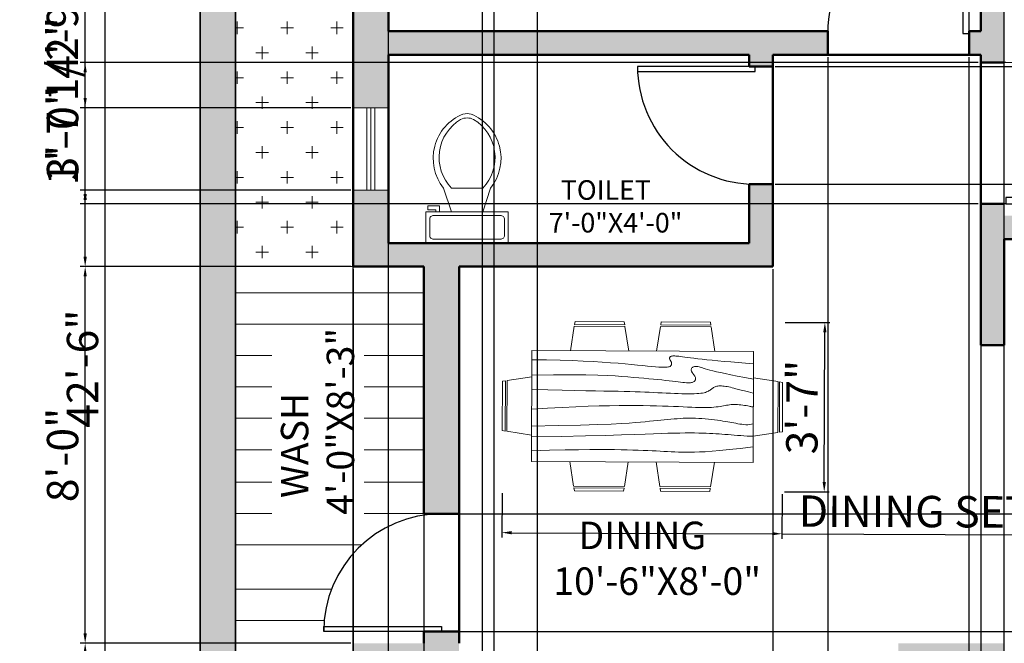
# Model space of a CAD drawing. Units: inches. Extents: x 1369 to 1844, y 2136 to 2743.
# Tile 2 of 4: x 1369 to 1620, y 2358 to 2517. Entities that reach past the tile are written whole.
import ezdxf

# ---------------------------------------------------------------- set-up
doc = ezdxf.new("R2010")
doc.units = ezdxf.units.IN
for name, color, linetype, lineweight in [('A-ANNO-DIMS', 2, 'Continuous', 18), ('A-AREA-IDEN', 7, 'Continuous', 25), ('A-DOOR', 4, 'Continuous', 25), ('A-FLOR-FIXT', 9, 'Continuous', 20), ('A-FLOR-PATT', 9, 'Continuous', 13), ('A-FURN', 8, 'Continuous', 18), ('A-WALL', 7, 'Continuous', 50), ('C-PROP', 7, 'Continuous', 35), ('L-PLNT', 3, 'Continuous', 18)]:
    doc.layers.add(name, color=color, linetype=linetype, lineweight=lineweight)
for name, color, linetype, lineweight, true_color in [('A-GLAZ', 244, 'Continuous', 20, 0x991b1e), ('A-WALL-PATT', 251, 'Continuous', 13, 0x636466), ('C-PROP-PATT', 251, 'Continuous', 13, 0x636466), ('L-PLNT-PATT', 116, 'Continuous', 13, 0x136734)]:
    doc.layers.add(name, color=color, linetype=linetype, lineweight=lineweight, true_color=true_color)
doc.styles.get("Standard").update_dxf_attribs({"font": 'arial.ttf'})
doc.dimstyles.new('ISO-25', dxfattribs={"dimtxt": 8, "dimasz": 2.5, "dimexe": 1.25, "dimexo": 0.625, "dimtad": 1, "dimlunit": 3, "dimtxsty": 'Standard', "dimcen": 2.5, "dimadec": 0, "dimazin": 0, "dimtfac": 1, "dimtmove": 0, "dimatfit": 3, "dimfxl": 1, "dimarcsym": 0})

# ---------------------------------------------------------------- blocks, each defined once
blk = doc.blocks.new('*U2')
for p, q in [((0, 0), (0, -6)), ((-40, 0), (-40, -6))]:
    blk.add_line(p, q)
blk.add_lwpolyline([(0, 0), (0, 40), (-1.75, 40), (-1.75, 0)], close=True)
blk.add_arc((0, 0), 40, 90, 180)
blk = doc.blocks.new('*U3')
for p, q in [((0, 0), (0, 6)), ((40, 0), (40, 6))]:
    blk.add_line(p, q)
blk.add_lwpolyline([(0, 0), (0, -40), (1.75, -40), (1.75, 0)], close=True)
blk.add_arc((0, 0), 40, 270, 360)
blk = doc.blocks.new('*U5')
for p, q in [((-40, 0), (-40, 6)), ((0, 0), (0, 6))]:
    blk.add_line(p, q)
blk.add_lwpolyline([(0, 0), (0, -40), (-1.75, -40), (-1.75, 0)], close=True)
blk.add_arc((0, 0), 40, 180, 270)
blk = doc.blocks.new('*U8')
for p, q in [((9.5, -6), (9.5, -2)), ((-10, -8.5), (-8, -8.5)), ((-10, -9.5), (-10, -8.5)), ((-7, -9.5), (-10, -9.5)), ((-8, -8.5), (-8, -8)), ((-7, -8), (-7, -9.5)), ((-4, -8), (-6, -14)), ((4, -8), (6, -14)), ((4, -14), (-4, -14))]:
    blk.add_line(p, q)
blk.add_lwpolyline([(10.5, -8), (10.5, 0), (-10.5, 0), (-10.5, -8)], close=True)
for points in [[(-9.5, -2), (-9.5, -6)], [(8.5, -1), (-8.5, -1)], [(-8.5, -7), (8.5, -7)]]:
    blk.add_lwpolyline(points)
for centre, radius, start, end in [((-8.62, -1.88), 0.884, 81.8699, 188.1301), ((8.62, -1.88), 0.884, 351.8699, 98.1301), ((-8.62, -6.12), 0.884, 171.8699, 278.1301), ((8.62, -6.12), 0.884, 261.8699, 8.1301), ((3.52, -21.58), 12.17, 141.4691, 247.9714), ((4.2, -21.82), 11.33, 136.3677, 238.9468), ((-3.52, -21.58), 12.17, 292.0284, 38.5307), ((-4.2, -21.82), 11.33, 301.053, 43.6321), ((0, -27.88), 4, 245.7318, 294.2682), ((0, -29), 4, 254.8605, 285.1395)]:
    blk.add_arc(centre, radius, start, end)
blk = doc.blocks.new('Dining Set - 36 x 72 in.')
for p, q in [((-22.2343, 26.00059), (-23.4847, 17.99762)), ((-22.2304, 26), (-5.7608, 26)), ((-22, 27.5), (-22.1562, 26.50042)), ((-5.8416, 26.5), (-22.1534, 26.5)), ((-22, 27.5), (-6, 27.5)), ((-5.8437, 26.49966), (-6, 27.5)), ((-4.5152, 17.99762), (-5.7655, 25.99926)), ((5.7657, 26.00059), (4.5153, 17.99762)), ((5.7696, 26), (22.2392, 26)), ((6, 27.5), (5.8438, 26.50042)), ((22.1584, 26.5), (5.8466, 26.5)), ((6, 27.5), (22, 27.5)), ((22.1563, 26.49966), (22, 27.5)), ((23.4848, 17.99762), (22.2345, 25.99926)), ((36, 18), (-36, 18)), ((-36, 18), (-36, -18)), ((36, -18), (36, 18)), ((-45.5, 8), (-44.5004, 8.15617)), ((-45.5, 8), (-45.5, -8)), ((-44.5, -8.15843), (-44.5, 8.15338)), ((-44.0006, 8.23428), (-35.9976, 9.48474)), ((-44, 8.23041), (-44, -8.23915)), ((44.0006, 8.23428), (35.9976, 9.48474)), ((44, 8.23041), (44, -8.23915)), ((44.5, -8.15843), (44.5, 8.15338)), ((45.5, 8), (44.5005, 8.15617)), ((45.5, 8), (45.5, -8)), ((-44.4997, -8.15631), (-45.5, -8)), ((-35.9976, -9.48476), (-43.9993, -8.2345)), ((35.9976, -9.48476), (43.9993, -8.2345)), ((44.4997, -8.15631), (45.5, -8)), ((-36, -18), (36, -18)), ((-22.2343, -26.0006), (-23.4847, -17.99762)), ((-4.5152, -17.99762), (-5.7655, -25.99928)), ((5.7657, -26.0006), (4.5153, -17.99762)), ((23.4848, -17.99762), (22.2345, -25.99928)), ((-22.2304, -26), (-5.7608, -26)), ((-22, -27.5), (-22.1562, -26.50044)), ((-5.8416, -26.5), (-22.1534, -26.5)), ((-22, -27.5), (-6, -27.5)), ((-5.8437, -26.49967), (-6, -27.5)), ((5.7696, -26), (22.2392, -26)), ((6, -27.5), (5.8438, -26.50044)), ((22.1584, -26.5), (5.8466, -26.5)), ((6, -27.5), (22, -27.5)), ((22.1563, -26.49967), (22, -27.5))]:
    blk.add_line(p, q)
for points in [[(-36, 15), (-31.1772, 14.97754), (-26.8079, 14.91406), (-22.8538, 14.81543), (-19.276, 14.6875), (-16.0362, 14.53613), (-13.0957, 14.36718), (-10.4159, 14.18652), (-7.9583, 14), (-5.6904, 13.81315), (-3.6035, 13.63021), (-1.6954, 13.45508), (0.0365, 13.29166), (1.5945, 13.14388), (2.9811, 13.01562), (4.1988, 12.9108), (5.25, 12.83333), (6.1393, 12.78613), (6.8802, 12.76823), (7.4883, 12.77767), (7.9792, 12.8125), (8.3685, 12.87077), (8.6719, 12.95052), (8.9049, 13.0498), (9.0833, 13.16666), (9.2205, 13.29899), (9.3216, 13.44401), (9.3895, 13.59879), (9.4271, 13.76041), (9.4373, 13.92594), (9.4232, 14.09245), (9.3875, 14.257), (9.3333, 14.41666), (9.2638, 14.56917), (9.1836, 14.71484), (9.0975, 14.85465), (9.0104, 14.98958), (8.9272, 15.1206), (8.8529, 15.2487), (8.7922, 15.37483), (8.75, 15.5), (8.7305, 15.62467), (8.7344, 15.74739), (8.7617, 15.86621), (8.8125, 15.97916), (8.8867, 16.08431), (8.9844, 16.17968), (9.1055, 16.26334), (9.25, 16.33333), (9.4189, 16.38802), (9.6172, 16.42708), (9.8506, 16.45052), (10.125, 16.45833), (10.4463, 16.45052), (10.8203, 16.42708), (11.2529, 16.38802), (11.75, 16.33333), (12.3184, 16.26318), (12.9694, 16.17838), (13.7151, 16.07991), (14.5677, 15.96875), (15.5395, 15.84586), (16.6426, 15.71224), (17.8893, 15.56884), (19.2917, 15.41666), (20.859, 15.25667), (22.5879, 15.08984), (24.4721, 14.91715), (26.5052, 14.73958), (28.6809, 14.5581), (30.9929, 14.3737), (33.4347, 14.18733), (36, 14)], [(-36, 10), (-28.9766, 10.14274), (-23.1725, 10.20442), (-18.4241, 10.19775), (-14.5677, 10.13541), (-11.4399, 10.03011), (-8.877, 9.89453), (-6.7154, 9.74137), (-4.7917, 9.58333), (-2.9698, 9.43082), (-1.2246, 9.28515), (0.4415, 9.14534), (2.026, 9.01041), (3.5266, 8.87939), (4.9408, 8.7513), (6.266, 8.62516), (7.5, 8.5), (8.6411, 8.37549), (9.6914, 8.2539), (10.6538, 8.13818), (11.5312, 8.03125), (12.3267, 7.93603), (13.043, 7.85547), (13.6831, 7.79248), (14.25, 7.75), (14.7471, 7.7303), (15.1797, 7.73307), (15.5537, 7.75732), (15.875, 7.80208), (16.1494, 7.86637), (16.3828, 7.94922), (16.5811, 8.04964), (16.75, 8.16666), (16.8944, 8.29915), (17.0143, 8.44531), (17.1089, 8.60319), (17.1771, 8.77083), (17.218, 8.94629), (17.2305, 9.1276), (17.2137, 9.31282), (17.1667, 9.5), (17.0895, 9.6875), (16.987, 9.875), (16.8649, 10.0625), (16.7292, 10.25), (16.5856, 10.4375), (16.4401, 10.625), (16.2985, 10.8125), (16.1667, 11), (16.05, 11.18733), (15.9518, 11.3737), (15.8752, 11.5581), (15.8229, 11.73958), (15.798, 11.91715), (15.8034, 12.08984), (15.842, 12.25667), (15.9167, 12.41666), (16.0295, 12.56836), (16.1784, 12.70833), (16.3605, 12.83268), (16.5729, 12.9375), (16.8127, 13.01888), (17.0768, 13.07291), (17.3625, 13.0957), (17.6667, 13.08333), (17.9894, 13.03312), (18.3418, 12.94726), (18.7382, 12.82918), (19.1927, 12.68229), (19.7195, 12.51001), (20.3327, 12.31575), (21.0465, 12.10294), (21.875, 11.875), (22.8357, 11.63354), (23.959, 11.37304), (25.2786, 11.08618), (26.8282, 10.76562), (28.6414, 10.40405), (30.752, 9.99414), (33.1936, 9.52856), (36, 9)], [(-36, 5.5), (-30.7157, 5.3348), (-26.069, 5.20963), (-21.9946, 5.11767), (-18.4271, 5.05208), (-15.3009, 5.00602), (-12.5508, 4.97265), (-10.1112, 4.94515), (-7.9167, 4.91666), (-5.909, 4.88167), (-4.0586, 4.83984), (-2.3429, 4.79215), (-0.7396, 4.73958), (0.7739, 4.6831), (2.22, 4.6237), (3.6213, 4.56233), (5, 4.5), (6.373, 4.43782), (7.7344, 4.3776), (9.0723, 4.32129), (10.375, 4.27083), (11.6309, 4.22819), (12.8281, 4.19531), (13.9551, 4.17415), (15, 4.16666), (15.954, 4.17448), (16.819, 4.19791), (17.6001, 4.23698), (18.3021, 4.29166), (18.9299, 4.36198), (19.4883, 4.44791), (19.9823, 4.54948), (20.4167, 4.66666), (20.7969, 4.79899), (21.1302, 4.94401), (21.4245, 5.09879), (21.6875, 5.26041), (21.9271, 5.42594), (22.1511, 5.59245), (22.3672, 5.757), (22.5834, 5.91666), (22.8065, 6.06868), (23.0404, 6.21093), (23.2879, 6.34147), (23.5521, 6.45833), (23.8358, 6.55957), (24.142, 6.64323), (24.4735, 6.70735), (24.8334, 6.75), (25.2235, 6.76969), (25.642, 6.76692), (26.0858, 6.74267), (26.5521, 6.69791), (27.0379, 6.63362), (27.5404, 6.55078), (28.0565, 6.45036), (28.5834, 6.33333), (29.1242, 6.19987), (29.7071, 6.04687), (30.3661, 5.87044), (31.1354, 5.66666), (32.0493, 5.43164), (33.142, 5.16146), (34.4475, 4.85221), (36, 4.5)], [(-36, -1), (-30.7915, -0.6591), (-26.0195, -0.38216), (-21.6519, -0.16284), (-17.6563, 0.00521), (-14.0005, 0.12833), (-10.6523, 0.21289), (-7.5796, 0.26522), (-4.75, 0.29166), (-2.134, 0.29793), (0.2878, 0.28711), (2.5317, 0.26163), (4.6146, 0.22396), (6.5529, 0.17651), (8.3633, 0.12174), (10.0623, 0.06209), (11.6667, 0), (13.1899, -0.06201), (14.6341, -0.1211), (15.9982, -0.17432), (17.2813, -0.21875), (18.4823, -0.25147), (19.6003, -0.26953), (20.6343, -0.27002), (21.5834, -0.25), (22.4481, -0.20768), (23.2357, -0.14584), (23.9549, -0.06836), (24.6146, 0.02083), (25.2235, 0.11784), (25.7904, 0.21875), (26.3241, 0.31966), (26.8334, 0.41666), (27.3265, 0.50618), (27.8099, 0.58593), (28.2894, 0.65397), (28.7709, 0.70833), (29.2601, 0.74707), (29.763, 0.76823), (30.2855, 0.76985), (30.8334, 0.75), (31.4088, 0.70784), (31.9994, 0.64713), (32.589, 0.57275), (33.1615, 0.48958), (33.7008, 0.4025), (34.1908, 0.3164), (34.6153, 0.23616), (34.9584, 0.16666), (35.2099, 0.11165), (35.3848, 0.07031), (35.504, 0.04069), (35.5886, 0.02083), (35.6594, 0.00879), (35.7377, 0.0026), (35.8442, 0.00032), (36, 0)], [(-36, -6.5), (-27.1843, -6.31267), (-20.084, -6.1263), (-14.469, -5.9419), (-10.1094, -5.76042), (-6.7752, -5.58285), (-4.2363, -5.41016), (-2.2629, -5.24333), (-0.625, -5.08334), (0.8708, -4.93099), (2.2715, -4.78646), (3.5872, -4.64974), (4.8281, -4.52084), (6.0046, -4.39974), (7.127, -4.28646), (8.2053, -4.18099), (9.25, -4.08334), (10.2705, -3.99382), (11.2734, -3.91407), (12.2647, -3.84603), (13.25, -3.79167), (14.2354, -3.75293), (15.2266, -3.73177), (16.2295, -3.73015), (17.25, -3.75), (18.2912, -3.79248), (19.3451, -3.85547), (20.4009, -3.93604), (21.4479, -4.03125), (22.4754, -4.13819), (23.4727, -4.25391), (24.4289, -4.37549), (25.3334, -4.5), (26.1785, -4.62492), (26.9694, -4.74935), (27.7145, -4.87281), (28.4219, -4.99479), (29.1, -5.11483), (29.7572, -5.23242), (30.4016, -5.34709), (31.0417, -5.45834), (31.6837, -5.56437), (32.3262, -5.65821), (32.9658, -5.73153), (33.599, -5.77604), (34.2224, -5.78345), (34.8327, -5.74545), (35.4264, -5.65373), (36, -5.5)], [(-36, -10), (-26.4022, -9.81299), (-18.4675, -9.62891), (-11.9839, -9.45069), (-6.7396, -9.28125), (-2.5226, -9.12354), (0.8789, -8.98047), (3.6769, -8.85498), (6.0833, -8.75), (8.2767, -8.66765), (10.3021, -8.60677), (12.1712, -8.56543), (13.8958, -8.54167), (15.4876, -8.53353), (16.9583, -8.53907), (18.3197, -8.55632), (19.5834, -8.58334), (20.7616, -8.61841), (21.8685, -8.66081), (22.9188, -8.71004), (23.9271, -8.76563), (24.9081, -8.82707), (25.8763, -8.89388), (26.8465, -8.96558), (27.8334, -9.04167), (28.8474, -9.12118), (29.8828, -9.20117), (30.93, -9.27824), (31.9792, -9.34896), (33.0205, -9.40991), (34.0443, -9.45768), (35.0407, -9.48885), (36, -9.5)], [(-36, -14.5), (-30.0881, -14.33513), (-25.0332, -14.21224), (-20.7312, -14.12647), (-17.0781, -14.07292), (-13.97, -14.04671), (-11.3027, -14.04297), (-8.9724, -14.05681), (-6.875, -14.08334), (-4.9224, -14.11833), (-3.0905, -14.16016), (-1.3709, -14.20785), (0.2448, -14.26042), (1.7647, -14.3169), (3.1973, -14.3763), (4.5507, -14.43767), (5.8333, -14.5), (7.0554, -14.5621), (8.235, -14.62175), (9.3922, -14.67652), (10.5469, -14.72396), (11.7192, -14.76164), (12.929, -14.78711), (14.1965, -14.79794), (15.5417, -14.79167), (16.9933, -14.76424), (18.6152, -14.70508), (20.4804, -14.60197), (22.6615, -14.44271), (25.2312, -14.21509), (28.2624, -13.9069), (31.8277, -13.50594), (36, -13)]]:
    blk.add_lwpolyline(points)
blk = doc.blocks.new('*D12')
at = {"layer": 'A-ANNO-DIMS', "color": 0, "lineweight": -2, "transparency": 16777216}
for p, q in [((1413.89, 2682.76), (1389.03, 2682.76)), ((1390.28, 2175.26), (1390.28, 2680.26)), ((1413.89, 2172.76), (1389.03, 2172.76))]:
    blk.add_line(p, q, dxfattribs=at)
at = {"layer": 'A-ANNO-DIMS', "color": 0, "transparency": 16777216}
for points in [[(1389.86, 2680.26), (1390.69, 2680.26), (1390.28, 2682.76)], [(1389.86, 2175.26), (1390.69, 2175.26), (1390.28, 2172.76)]]:
    blk.add_solid(points, dxfattribs=at)
at = {"layer": 'Defpoints', "color": 0, "transparency": 16777216}
for p in [(1390.28, 2682.76), (1414.51, 2682.76), (1414.51, 2172.76)]:
    blk.add_point(p, dxfattribs=at)
at = {"layer": 'A-ANNO-DIMS', "color": 0, "transparency": 16777216, "insert": (1385.57, 2427.76), "char_height": 8, "attachment_point": 5, "rotation": 90}
blk.add_mtext('42\'-6"', dxfattribs=at)
blk = doc.blocks.new('WIN-21IN')
for p, q in [((3.5, 21), (3.5, 0)), ((4.5, 21), (4.5, 0)), ((5.5, 21), (5.5, 0))]:
    blk.add_line(p, q)
blk.add_lwpolyline([(0, 21), (9, 21), (9, 0), (0, 0)], close=True)
blk = doc.blocks.new('*D24')
at = {"layer": 'A-ANNO-DIMS', "color": 0, "lineweight": -2, "transparency": 16777216}
for p, q in [((1491.47, 2396.04), (1491.42, 2384.71)), ((1562.89, 2395.76), (1562.84, 2384.42)), ((1493.93, 2385.95), (1560.35, 2385.68)), ((1562.85, 2385.67), (1679.38, 2385.22))]:
    blk.add_line(p, q, dxfattribs=at)
at = {"layer": 'A-ANNO-DIMS', "color": 0, "transparency": 16777216}
for points in [[(1493.93, 2386.36), (1493.93, 2385.53), (1491.43, 2385.96)], [(1560.35, 2386.1), (1560.35, 2385.27), (1562.85, 2385.67)]]:
    blk.add_solid(points, dxfattribs=at)
at = {"layer": 'Defpoints', "color": 0, "transparency": 16777216}
for p in [(1491.47, 2396.67), (1562.89, 2396.39), (1562.85, 2385.67)]:
    blk.add_point(p, dxfattribs=at)
at = {"layer": 'A-ANNO-DIMS', "color": 0, "transparency": 16777216, "insert": (1622.38, 2390.2), "char_height": 8, "attachment_point": 5, "rotation": 359.7742}
blk.add_mtext('DINING SET 5\'-11 1/2"', dxfattribs=at)
blk = doc.blocks.new('*D25')
at = {"layer": 'A-ANNO-DIMS', "color": 0, "lineweight": -2, "transparency": 16777216}
for p, q in [((1563.69, 2439.55), (1575.02, 2439.51)), ((1573.61, 2398.85), (1573.76, 2437.01)), ((1563.52, 2396.38), (1574.85, 2396.34))]:
    blk.add_line(p, q, dxfattribs=at)
at = {"layer": 'A-ANNO-DIMS', "color": 0, "transparency": 16777216}
for points in [[(1573.35, 2437.01), (1574.18, 2437.01), (1573.77, 2439.51)], [(1573.2, 2398.85), (1574.03, 2398.84), (1573.6, 2396.35)]]:
    blk.add_solid(points, dxfattribs=at)
at = {"layer": 'Defpoints', "color": 0, "transparency": 16777216}
for p in [(1563.06, 2439.55), (1573.77, 2439.51), (1562.89, 2396.39)]:
    blk.add_point(p, dxfattribs=at)
at = {"layer": 'A-ANNO-DIMS', "color": 0, "transparency": 16777216, "insert": (1568.98, 2417.95), "char_height": 8, "attachment_point": 5, "rotation": 89.7742}
blk.add_mtext('3\'-7"', dxfattribs=at)
blk = doc.blocks.new('*D37')
at = {"layer": 'A-ANNO-DIMS', "color": 0, "lineweight": -2, "transparency": 16777216}
for p, q in [((1452.89, 2357.76), (1383.96, 2357.76)), ((1385.21, 2261.26), (1385.21, 2355.26)), ((1452.89, 2258.76), (1383.96, 2258.76))]:
    blk.add_line(p, q, dxfattribs=at)
at = {"layer": 'A-ANNO-DIMS', "color": 0, "transparency": 16777216}
for points in [[(1384.79, 2355.26), (1385.63, 2355.26), (1385.21, 2357.76)], [(1384.79, 2261.26), (1385.63, 2261.26), (1385.21, 2258.76)]]:
    blk.add_solid(points, dxfattribs=at)
at = {"layer": 'Defpoints', "color": 0, "transparency": 16777216}
for p in [(1385.21, 2357.76), (1453.51, 2357.76), (1453.51, 2258.76)]:
    blk.add_point(p, dxfattribs=at)
at = {"layer": 'A-ANNO-DIMS', "color": 0, "transparency": 16777216, "insert": (1380.5, 2308.26), "char_height": 8, "attachment_point": 5, "rotation": 90}
blk.add_mtext('8\'-3"', dxfattribs=at)
blk = doc.blocks.new('*D38')
at = {"layer": 'A-ANNO-DIMS', "color": 0, "lineweight": -2, "transparency": 16777216}
for p, q in [((1452.89, 2453.76), (1383.96, 2453.76)), ((1385.21, 2360.26), (1385.21, 2451.26)), ((1452.89, 2357.76), (1383.96, 2357.76))]:
    blk.add_line(p, q, dxfattribs=at)
at = {"layer": 'A-ANNO-DIMS', "color": 0, "transparency": 16777216}
for points in [[(1384.79, 2451.26), (1385.63, 2451.26), (1385.21, 2453.76)], [(1384.79, 2360.26), (1385.63, 2360.26), (1385.21, 2357.76)]]:
    blk.add_solid(points, dxfattribs=at)
at = {"layer": 'Defpoints', "color": 0, "transparency": 16777216}
for p in [(1385.21, 2453.76), (1453.51, 2453.76), (1453.51, 2357.76)]:
    blk.add_point(p, dxfattribs=at)
at = {"layer": 'A-ANNO-DIMS', "color": 0, "transparency": 16777216, "insert": (1380.5, 2405.76), "char_height": 8, "attachment_point": 5, "rotation": 90}
blk.add_mtext('8\'-0"', dxfattribs=at)
blk = doc.blocks.new('*D39')
at = {"layer": 'A-ANNO-DIMS', "color": 0, "lineweight": -2, "transparency": 16777216}
for p, q in [((1385.21, 2473.26), (1385.21, 2516.16)), ((1452.89, 2473.26), (1383.96, 2473.26)), ((1385.21, 2456.26), (1385.21, 2470.76)), ((1452.89, 2453.76), (1383.96, 2453.76))]:
    blk.add_line(p, q, dxfattribs=at)
at = {"layer": 'A-ANNO-DIMS', "color": 0, "transparency": 16777216}
for points in [[(1384.79, 2470.76), (1385.63, 2470.76), (1385.21, 2473.26)], [(1384.79, 2456.26), (1385.63, 2456.26), (1385.21, 2453.76)]]:
    blk.add_solid(points, dxfattribs=at)
at = {"layer": 'Defpoints', "color": 0, "transparency": 16777216}
for p in [(1385.21, 2473.26), (1453.51, 2473.26), (1453.51, 2453.76)]:
    blk.add_point(p, dxfattribs=at)
at = {"layer": 'A-ANNO-DIMS', "color": 0, "transparency": 16777216, "insert": (1380.45, 2495.96), "char_height": 8, "attachment_point": 5, "rotation": 90}
blk.add_mtext('1\'-7 1/2"', dxfattribs=at)
blk = doc.blocks.new('*D40')
at = {"layer": 'A-ANNO-DIMS', "color": 0, "lineweight": -2, "transparency": 16777216}
for p, q in [((1452.89, 2551.88), (1383.96, 2551.88)), ((1385.21, 2496.76), (1385.21, 2549.38)), ((1452.89, 2494.26), (1383.96, 2494.26))]:
    blk.add_line(p, q, dxfattribs=at)
at = {"layer": 'A-ANNO-DIMS', "color": 0, "transparency": 16777216}
for points in [[(1384.79, 2549.38), (1385.63, 2549.38), (1385.21, 2551.88)], [(1384.79, 2496.76), (1385.63, 2496.76), (1385.21, 2494.26)]]:
    blk.add_solid(points, dxfattribs=at)
at = {"layer": 'Defpoints', "color": 0, "transparency": 16777216}
for p in [(1385.21, 2551.88), (1453.51, 2551.88), (1453.51, 2494.26)]:
    blk.add_point(p, dxfattribs=at)
at = {"layer": 'A-ANNO-DIMS', "color": 0, "transparency": 16777216, "insert": (1380.45, 2523.07), "char_height": 8, "attachment_point": 5, "rotation": 90}
blk.add_mtext('4\'-9 1/2"', dxfattribs=at)
blk = doc.blocks.new('*D42')
at = {"layer": 'A-ANNO-DIMS', "color": 0, "lineweight": -2, "transparency": 16777216}
for p, q in [((1453.51, 2453.13), (1453.51, 2142.21)), ((1471.51, 2453.13), (1471.51, 2142.21)), ((1456.01, 2143.46), (1469.01, 2143.46)), ((1471.51, 2143.46), (1495.77, 2143.46))]:
    blk.add_line(p, q, dxfattribs=at)
at = {"layer": 'A-ANNO-DIMS', "color": 0, "transparency": 16777216}
for points in [[(1456.01, 2143.87), (1456.01, 2143.04), (1453.51, 2143.46)], [(1469.01, 2143.87), (1469.01, 2143.04), (1471.51, 2143.46)]]:
    blk.add_solid(points, dxfattribs=at)
at = {"layer": 'Defpoints', "color": 0, "transparency": 16777216}
for p in [(1453.51, 2453.76), (1471.51, 2453.76), (1471.51, 2143.46)]:
    blk.add_point(p, dxfattribs=at)
at = {"layer": 'A-ANNO-DIMS', "color": 0, "transparency": 16777216, "insert": (1484.89, 2148.17), "char_height": 8, "attachment_point": 5}
blk.add_mtext('1\'-6"', dxfattribs=at)
blk = doc.blocks.new('*D45')
at = {"layer": 'A-ANNO-DIMS', "color": 0, "lineweight": -2, "transparency": 16777216}
for p, q in [((1619.51, 2326.38), (1619.51, 2734.31)), ((1636.5, 2326.38), (1636.5, 2734.31)), ((1622.01, 2733.06), (1634, 2733.06)), ((1636.5, 2733.06), (1660.77, 2733.06))]:
    blk.add_line(p, q, dxfattribs=at)
at = {"layer": 'A-ANNO-DIMS', "color": 0, "transparency": 16777216}
for points in [[(1622.01, 2733.47), (1622.01, 2732.64), (1619.51, 2733.06)], [(1634, 2733.47), (1634, 2732.64), (1636.5, 2733.06)]]:
    blk.add_solid(points, dxfattribs=at)
at = {"layer": 'Defpoints', "color": 0, "transparency": 16777216}
for p in [(1636.5, 2733.06), (1619.51, 2325.76), (1636.5, 2325.76)]:
    blk.add_point(p, dxfattribs=at)
at = {"layer": 'A-ANNO-DIMS', "color": 0, "transparency": 16777216, "insert": (1649.88, 2737.77), "char_height": 8, "attachment_point": 5}
blk.add_mtext('1\'-5"', dxfattribs=at)
blk = doc.blocks.new('*D49')
at = {"layer": 'A-ANNO-DIMS', "color": 0, "lineweight": -2, "transparency": 16777216}
for p, q in [((1574.51, 2507.13), (1574.51, 2142.21)), ((1610.51, 2507.13), (1610.51, 2142.21)), ((1577.01, 2143.46), (1608.01, 2143.46))]:
    blk.add_line(p, q, dxfattribs=at)
at = {"layer": 'A-ANNO-DIMS', "color": 0, "transparency": 16777216}
for points in [[(1577.01, 2143.87), (1577.01, 2143.04), (1574.51, 2143.46)], [(1608.01, 2143.87), (1608.01, 2143.04), (1610.51, 2143.46)]]:
    blk.add_solid(points, dxfattribs=at)
at = {"layer": 'Defpoints', "color": 0, "transparency": 16777216}
for p in [(1574.51, 2507.76), (1610.51, 2507.76), (1610.51, 2143.46)]:
    blk.add_point(p, dxfattribs=at)
at = {"layer": 'A-ANNO-DIMS', "color": 0, "transparency": 16777216, "insert": (1592.51, 2148.17), "char_height": 8, "attachment_point": 5}
blk.add_mtext('3\'-0"', dxfattribs=at)
blk = doc.blocks.new('*D50')
at = {"layer": 'A-ANNO-DIMS', "color": 0, "lineweight": -2, "transparency": 16777216}
for p, q in [((1612.89, 2505.76), (1383.96, 2505.76)), ((1385.21, 2472.26), (1385.21, 2503.26)), ((1612.89, 2469.76), (1383.96, 2469.76))]:
    blk.add_line(p, q, dxfattribs=at)
at = {"layer": 'A-ANNO-DIMS', "color": 0, "transparency": 16777216}
for points in [[(1384.79, 2503.26), (1385.63, 2503.26), (1385.21, 2505.76)], [(1384.79, 2472.26), (1385.63, 2472.26), (1385.21, 2469.76)]]:
    blk.add_solid(points, dxfattribs=at)
at = {"layer": 'Defpoints', "color": 0, "transparency": 16777216}
for p in [(1385.21, 2505.76), (1613.51, 2505.76), (1613.51, 2469.76)]:
    blk.add_point(p, dxfattribs=at)
at = {"layer": 'A-ANNO-DIMS', "color": 0, "transparency": 16777216, "insert": (1380.5, 2487.76), "char_height": 8, "attachment_point": 5, "rotation": 90}
blk.add_mtext('3\'-0"', dxfattribs=at)
blk = doc.blocks.new('*D51')
at = {"layer": 'A-ANNO-DIMS', "color": 0, "lineweight": -2, "transparency": 16777216}
for p, q in [((1561.14, 2504.76), (1838.06, 2504.76)), ((1836.81, 2477.26), (1836.81, 2502.26)), ((1561.14, 2474.76), (1838.06, 2474.76))]:
    blk.add_line(p, q, dxfattribs=at)
at = {"layer": 'A-ANNO-DIMS', "color": 0, "transparency": 16777216}
for points in [[(1836.39, 2502.26), (1837.23, 2502.26), (1836.81, 2504.76)], [(1836.39, 2477.26), (1837.23, 2477.26), (1836.81, 2474.76)]]:
    blk.add_solid(points, dxfattribs=at)
at = {"layer": 'Defpoints', "color": 0, "transparency": 16777216}
for p in [(1560.51, 2504.76), (1836.81, 2504.76), (1560.51, 2474.76)]:
    blk.add_point(p, dxfattribs=at)
at = {"layer": 'A-ANNO-DIMS', "color": 0, "transparency": 16777216, "insert": (1832.1, 2489.76), "char_height": 8, "attachment_point": 5, "rotation": 90}
blk.add_mtext('2\'-6"', dxfattribs=at)
blk = doc.blocks.new('*D52')
at = {"layer": 'A-ANNO-DIMS', "color": 0, "lineweight": -2, "transparency": 16777216}
for p, q in [((1472.14, 2390.76), (1838.06, 2390.76)), ((1836.81, 2363.26), (1836.81, 2388.26)), ((1472.14, 2360.76), (1838.06, 2360.76))]:
    blk.add_line(p, q, dxfattribs=at)
at = {"layer": 'A-ANNO-DIMS', "color": 0, "transparency": 16777216}
for points in [[(1836.39, 2388.26), (1837.23, 2388.26), (1836.81, 2390.76)], [(1836.39, 2363.26), (1837.23, 2363.26), (1836.81, 2360.76)]]:
    blk.add_solid(points, dxfattribs=at)
at = {"layer": 'Defpoints', "color": 0, "transparency": 16777216}
for p in [(1471.51, 2390.76), (1836.81, 2390.76), (1471.51, 2360.76)]:
    blk.add_point(p, dxfattribs=at)
at = {"layer": 'A-ANNO-DIMS', "color": 0, "transparency": 16777216, "insert": (1832.1, 2375.76), "char_height": 8, "attachment_point": 5, "rotation": 90}
blk.add_mtext('2\'-6"', dxfattribs=at)
blk = doc.blocks.new('*D53')
at = {"layer": 'A-ANNO-DIMS', "color": 0, "lineweight": -2, "transparency": 16777216}
for p, q in [((1613.51, 2469.13), (1613.51, 2142.21)), ((1560.51, 2453.13), (1560.51, 2142.21)), ((1563.01, 2143.46), (1611.01, 2143.46))]:
    blk.add_line(p, q, dxfattribs=at)
at = {"layer": 'A-ANNO-DIMS', "color": 0, "transparency": 16777216}
for points in [[(1563.01, 2143.87), (1563.01, 2143.04), (1560.51, 2143.46)], [(1611.01, 2143.87), (1611.01, 2143.04), (1613.51, 2143.46)]]:
    blk.add_solid(points, dxfattribs=at)
at = {"layer": 'Defpoints', "color": 0, "transparency": 16777216}
for p in [(1613.51, 2469.76), (1560.51, 2453.76), (1613.51, 2143.46)]:
    blk.add_point(p, dxfattribs=at)
at = {"layer": 'A-ANNO-DIMS', "color": 0, "transparency": 16777216, "insert": (1587.01, 2148.15), "char_height": 8, "attachment_point": 5}
blk.add_mtext('4\'-5"', dxfattribs=at)
blk = doc.blocks.new('*D54')
at = {"layer": 'A-ANNO-DIMS', "color": 0, "lineweight": -2, "transparency": 16777216}
for p, q in [((1462.51, 2268.38), (1462.51, 2734.31)), ((1486.51, 2292.38), (1486.51, 2734.31)), ((1465.01, 2733.06), (1484.01, 2733.06))]:
    blk.add_line(p, q, dxfattribs=at)
at = {"layer": 'A-ANNO-DIMS', "color": 0, "transparency": 16777216}
for points in [[(1465.01, 2733.47), (1465.01, 2732.64), (1462.51, 2733.06)], [(1484.01, 2733.47), (1484.01, 2732.64), (1486.51, 2733.06)]]:
    blk.add_solid(points, dxfattribs=at)
at = {"layer": 'Defpoints', "color": 0, "transparency": 16777216}
for p in [(1486.51, 2733.06), (1486.51, 2291.76), (1462.51, 2267.76)]:
    blk.add_point(p, dxfattribs=at)
at = {"layer": 'A-ANNO-DIMS', "color": 0, "transparency": 16777216, "insert": (1474.51, 2737.77), "char_height": 8, "attachment_point": 5}
blk.add_mtext('2\'-0"', dxfattribs=at)
blk = doc.blocks.new('*D55')
at = {"layer": 'A-ANNO-DIMS', "color": 0, "lineweight": -2, "transparency": 16777216}
for p, q in [((1453.51, 2179.38), (1453.51, 2734.31)), ((1489.51, 2179.38), (1489.51, 2734.31)), ((1456.01, 2733.06), (1487.01, 2733.06))]:
    blk.add_line(p, q, dxfattribs=at)
at = {"layer": 'A-ANNO-DIMS', "color": 0, "transparency": 16777216}
for points in [[(1456.01, 2733.47), (1456.01, 2732.64), (1453.51, 2733.06)], [(1487.01, 2733.47), (1487.01, 2732.64), (1489.51, 2733.06)]]:
    blk.add_solid(points, dxfattribs=at)
at = {"layer": 'Defpoints', "color": 0, "transparency": 16777216}
for p in [(1489.51, 2733.06), (1453.51, 2178.76), (1489.51, 2178.76)]:
    blk.add_point(p, dxfattribs=at)
at = {"layer": 'A-ANNO-DIMS', "color": 0, "transparency": 16777216, "insert": (1471.51, 2737.77), "char_height": 8, "attachment_point": 5}
blk.add_mtext('3\'-0"', dxfattribs=at)
blk = doc.blocks.new('*D56')
at = {"layer": 'A-ANNO-DIMS', "color": 0, "lineweight": -2, "transparency": 16777216}
for p, q in [((1489.51, 2222.38), (1489.51, 2734.31)), ((1500.51, 2222.38), (1500.51, 2734.31)), ((1492.01, 2733.06), (1498.01, 2733.06)), ((1500.51, 2733.06), (1531.74, 2733.06))]:
    blk.add_line(p, q, dxfattribs=at)
at = {"layer": 'A-ANNO-DIMS', "color": 0, "transparency": 16777216}
for points in [[(1492.01, 2733.47), (1492.01, 2732.64), (1489.51, 2733.06)], [(1498.01, 2733.47), (1498.01, 2732.64), (1500.51, 2733.06)]]:
    blk.add_solid(points, dxfattribs=at)
at = {"layer": 'Defpoints', "color": 0, "transparency": 16777216}
for p in [(1500.51, 2733.06), (1489.51, 2221.76), (1500.51, 2221.76)]:
    blk.add_point(p, dxfattribs=at)
at = {"layer": 'A-ANNO-DIMS', "color": 0, "transparency": 16777216, "insert": (1517.38, 2737.77), "char_height": 8, "attachment_point": 5}
blk.add_mtext('0\'-11"', dxfattribs=at)

msp = doc.modelspace()

# ---------------------------------------------------------------- hatches: boundary and pattern name
at = {"layer": 'A-WALL-PATT'}
h = msp.add_hatch(color=256, dxfattribs=at)
h.dxf.hatch_style = 1
h.paths.add_polyline_path([(1619.511, 2460.756), (1768.511, 2460.756), (1768.511, 2444.065), (1777.511, 2444.065), (1777.511, 2498.256), (1768.511, 2498.256), (1768.511, 2466.756), (1619.511, 2466.756), (1619.511, 2469.756), (1614.511, 2469.756), (1613.511, 2469.756), (1613.511, 2433.756), (1619.511, 2433.756)])
h.paths.add_polyline_path([(1480.511, 2453.756), (1560.511, 2453.756), (1560.511, 2474.756), (1556.011, 2474.756), (1554.511, 2474.756), (1554.511, 2459.756), (1462.511, 2459.756), (1462.511, 2473.256), (1453.511, 2473.256), (1453.511, 2453.756), (1471.511, 2453.756), (1471.511, 2390.756), (1480.511, 2390.756)])
h.paths.add_polyline_path([(1574.511, 2513.156), (1574.511, 2513.756), (1462.511, 2513.756), (1462.511, 2551.882), (1453.511, 2551.882), (1453.511, 2494.256), (1462.511, 2494.256), (1462.511, 2507.756), (1554.511, 2507.756), (1554.511, 2504.756), (1556.011, 2504.756), (1560.511, 2504.756), (1560.511, 2507.756), (1574.511, 2507.756)])
h.paths.add_polyline_path([(1462.511, 2351.756), (1480.511, 2351.756), (1480.511, 2357.756), (1480.511, 2360.756), (1476.011, 2360.756), (1471.511, 2360.756), (1471.511, 2357.756), (1453.511, 2357.756), (1453.511, 2258.756), (1508.011, 2258.756), (1508.011, 2267.756), (1462.511, 2267.756)])
h.paths.add_polyline_path([(1619.511, 2357.756), (1592.511, 2357.756), (1592.511, 2351.756), (1613.511, 2351.756), (1613.511, 2267.756), (1568.011, 2267.756), (1568.011, 2258.756), (1619.511, 2258.756), (1619.511, 2316.756), (1636.503, 2316.756), (1636.503, 2325.756), (1619.511, 2325.756)])
h.paths.add_polyline_path([(1717.511, 2323.956), (1717.511, 2325.756), (1696.503, 2325.756), (1696.503, 2316.756), (1717.511, 2316.756)])
h.paths.add_polyline_path([(1777.511, 2384.065), (1768.511, 2384.065), (1768.511, 2325.756), (1765.511, 2325.756), (1765.511, 2323.956), (1765.511, 2316.756), (1777.511, 2316.756)])
h.paths.add_polyline_path([(1777.511, 2652.756), (1731.511, 2652.756), (1731.511, 2643.756), (1768.511, 2643.756), (1768.511, 2595.756), (1673.511, 2595.756), (1673.511, 2598.756), (1672.011, 2598.756), (1667.511, 2598.756), (1667.511, 2595.756), (1613.511, 2595.756), (1613.511, 2513.756), (1610.511, 2513.756), (1610.511, 2513.156), (1610.511, 2507.756), (1613.511, 2507.756), (1613.511, 2505.756), (1619.511, 2505.756), (1619.511, 2589.756), (1768.511, 2589.756), (1768.511, 2558.256), (1777.511, 2558.256)])
h.paths.add_polyline_path([(1710.511, 2652.756), (1616.643, 2652.756), (1616.643, 2643.756), (1667.511, 2643.756), (1667.511, 2628.756), (1672.011, 2628.756), (1673.511, 2628.756), (1673.511, 2643.756), (1710.511, 2643.756)], flags=17)
h.paths.add_polyline_path([(1556.643, 2652.756), (1453.511, 2652.756), (1453.511, 2611.882), (1462.511, 2611.882), (1462.511, 2643.756), (1556.643, 2643.756)])
at = {"layer": 'C-PROP-PATT'}
h = msp.add_hatch(color=256, dxfattribs=at)
h.dxf.hatch_style = 1
h.paths.add_polyline_path([(1423.511, 2676.756), (1801.511, 2676.756), (1801.511, 2178.756), (1777.511, 2178.756), (1777.511, 2172.756), (1807.511, 2172.756), (1807.511, 2682.756), (1414.511, 2682.756), (1414.511, 2172.756), (1642.884, 2172.756), (1642.884, 2178.756), (1423.511, 2178.756)])
at = {"layer": 'L-PLNT-PATT'}
h = msp.add_hatch(dxfattribs=at)
h.set_pattern_fill('CROSS', color=256)
h.paths.add_polyline_path([(1453.511, 2652.756), (1777.511, 2652.756), (1788.511, 2652.756), (1788.511, 2178.756), (1801.511, 2178.756), (1801.511, 2676.756), (1423.511, 2676.756), (1423.511, 2453.756), (1453.511, 2453.756)])
h.paths.add_polyline_path([(1453.511, 2350.279), (1423.511, 2350.279), (1423.511, 2178.756), (1453.511, 2178.756), (1453.511, 2258.756)], flags=17)

# ---------------------------------------------------------------- linework, layer by layer
at = {"layer": 'A-FLOR-PATT'}
for p, q in [((1471.511, 2447.086), (1423.511, 2447.086)), ((1471.511, 2439.086), (1423.511, 2439.086)), ((1432.766, 2431.086), (1423.511, 2431.086)), ((1471.511, 2431.086), (1456.371, 2431.086)), ((1432.766, 2423.093), (1423.511, 2423.093)), ((1471.511, 2423.093), (1456.371, 2423.093)), ((1432.766, 2415.093), (1423.511, 2415.093)), ((1471.511, 2415.093), (1456.371, 2415.093)), ((1432.766, 2407.093), (1423.511, 2407.093)), ((1471.511, 2407.093), (1456.371, 2407.093)), ((1432.766, 2398.857), (1423.511, 2398.857)), ((1471.511, 2398.857), (1456.371, 2398.857)), ((1432.766, 2390.857), (1423.511, 2390.857)), ((1471.511, 2390.857), (1456.371, 2390.857)), ((1455.725, 2382.857), (1423.511, 2382.857)), ((1448.017, 2371.542), (1423.511, 2371.542)), ((1446.141, 2363.542), (1423.511, 2363.542))]:
    msp.add_line(p, q, dxfattribs=at)
at = {"layer": 'A-WALL'}
for p, q in [((1453.511, 2652.756), (1453.511, 2453.756)), ((1462.511, 2643.756), (1462.511, 2513.756)), ((1613.511, 2595.756), (1613.511, 2513.756)), ((1462.511, 2513.756), (1574.511, 2513.756)), ((1574.511, 2507.756), (1574.511, 2513.756)), ((1610.511, 2507.756), (1610.511, 2513.756)), ((1610.511, 2513.756), (1613.511, 2513.756)), ((1462.511, 2507.756), (1554.511, 2507.756)), ((1462.511, 2507.756), (1462.511, 2459.756)), ((1554.511, 2507.756), (1554.511, 2504.756)), ((1560.511, 2507.756), (1560.511, 2453.756)), ((1560.511, 2507.756), (1613.511, 2507.756)), ((1613.511, 2507.756), (1613.511, 2433.756)), ((1619.511, 2505.756), (1613.511, 2505.756)), ((1560.511, 2504.756), (1554.511, 2504.756)), ((1554.511, 2474.756), (1554.511, 2459.756)), ((1560.511, 2474.756), (1554.511, 2474.756)), ((1619.511, 2469.756), (1613.511, 2469.756)), ((1462.511, 2459.756), (1554.511, 2459.756)), ((1619.511, 2460.756), (1768.511, 2460.756)), ((1619.511, 2460.756), (1619.511, 2433.756)), ((1453.511, 2453.756), (1471.511, 2453.756)), ((1471.511, 2453.756), (1471.511, 2390.756)), ((1480.511, 2453.756), (1480.511, 2357.756)), ((1480.511, 2453.756), (1560.511, 2453.756)), ((1619.511, 2433.756), (1613.511, 2433.756)), ((1471.511, 2390.756), (1480.511, 2390.756)), ((1471.511, 2360.756), (1480.511, 2360.756)), ((1471.511, 2360.756), (1471.511, 2357.756))]:
    msp.add_line(p, q, dxfattribs=at)
at = {"layer": 'C-PROP'}
for p, q in [((1414.511, 2682.756), (1414.511, 2172.756)), ((1423.511, 2676.756), (1423.511, 2178.756))]:
    msp.add_line(p, q, dxfattribs=at)
at = {"layer": 'L-PLNT'}
msp.add_line((1423.511, 2453.756), (1453.511, 2453.756), dxfattribs=at)

# ---------------------------------------------------------------- block references
at = {"layer": 'A-DOOR', "xscale": 0.9, "yscale": 0.9, "zscale": 0.9}
msp.add_blockref('*U2', (1610.511, 2513.156), dxfattribs=at)
at = {"layer": 'A-DOOR', "rotation": 270}
for name, p, xscale, yscale, zscale in [('*U2', (1619.911, 2469.756), 0.9, 0.9, 0.9), ('*U3', (1556.011, 2504.756), 0.75, 0.75, 0.75), ('*U5', (1476.011, 2360.756), 0.75, 0.75, 0.75)]:
    msp.add_blockref(name, p, dxfattribs=dict(at, xscale=xscale, yscale=yscale, zscale=zscale))
at = {"layer": 'A-FLOR-FIXT', "xscale": -1, "rotation": 180}
msp.add_blockref('*U8', (1482.567, 2459.756), dxfattribs=at)
at = {"layer": 'A-FURN', "xscale": 0.784841063558616, "yscale": 0.784841063558616, "zscale": 0.784841063558616, "rotation": 359.7741561953044}
msp.add_blockref('Dining Set - 36 x 72 in.', (1527.265, 2418.111), dxfattribs=at)
at = {"layer": 'A-GLAZ'}
msp.add_blockref('WIN-21IN', (1453.511, 2473.256), dxfattribs=at)

# ---------------------------------------------------------------- texts
at = {"layer": 'A-AREA-IDEN', "attachment_point": 1}
for s, width, insert, char_height in [('  TOILET   7\'-0"X4\'-0"', 32.93692, (1503.403, 2475.783), 5), ('   DINING\\P10\'-6"X8\'-0"', 50.15129, (1504.541, 2388.763), 7)]:
    msp.add_mtext_dynamic_manual_height_columns(s, width=width, gutter_width=12.5, heights=[0], dxfattribs=dict(at, insert=insert, char_height=char_height))
at = {"layer": 'A-AREA-IDEN', "insert": (1435.099, 2390.49), "char_height": 7, "attachment_point": 1, "rotation": 90}
msp.add_mtext_dynamic_manual_height_columns('  WASH\\P4\'-0"X8\'-3"', width=45.96465, gutter_width=12.5, heights=[0], dxfattribs=at)

# ---------------------------------------------------------------- dimensions: what is measured, and where the dimension line sits
at = {"layer": 'A-ANNO-DIMS'}
for base, p1, p2, picture, middle in [((1489.511, 2733.056), (1453.511, 2178.756), (1489.511, 2178.756), '*D55', (1471.511, 2737.768)), ((1486.511, 2733.056), (1462.511, 2267.756), (1486.511, 2291.756), '*D54', (1474.511, 2737.766)), ((1500.511, 2733.056), (1489.511, 2221.756), (1500.511, 2221.756), '*D56', (1517.377, 2737.766)), ((1636.503, 2733.056), (1619.511, 2325.756), (1636.503, 2325.756), '*D45', (1649.884, 2737.766)), ((1610.511, 2143.456), (1574.511, 2507.756), (1610.511, 2507.756), '*D49', (1592.511, 2148.168)), ((1613.511, 2143.456), (1560.511, 2453.756), (1613.511, 2469.756), '*D53', (1587.011, 2148.149)), ((1471.511, 2143.456), (1453.511, 2453.756), (1471.511, 2453.756), '*D42', (1484.893, 2148.166))]:
    dim = msp.add_linear_dim(base=base, p1=p1, p2=p2, dimstyle='ISO-25', override={"dimdec": 1, "dimlfac": 1, "dimrnd": 0, "dimzin": 1, "dimdsep": 46, "dimlunit": 4, "dimfrac": 2}, dxfattribs=at)
    dim.commit()
    dim.dimension.update_dxf_attribs({"geometry": picture, "text_midpoint": middle})
for base, p1, p2, angle, override, picture, middle in [((1390.277, 2682.756), (1414.511, 2172.756), (1414.511, 2682.756), 90, {"dimclrd": 0, "dimclre": 0, "dimclrt": 0}, '*D12', (1385.567, 2427.756)), ((1385.211, 2551.882), (1453.511, 2494.256), (1453.511, 2551.882), 90, {"dimdec": 1, "dimlfac": 1, "dimrnd": 0, "dimzin": 1, "dimdsep": 46, "dimlunit": 4, "dimfrac": 2}, '*D40', (1380.45, 2523.069)), ((1385.211, 2473.256), (1453.511, 2453.756), (1453.511, 2473.256), 90, {"dimdec": 1, "dimlfac": 1, "dimrnd": 0, "dimzin": 1, "dimdsep": 46, "dimlunit": 4, "dimfrac": 2}, '*D39', (1380.45, 2495.958)), ((1385.211, 2505.756), (1613.511, 2469.756), (1613.511, 2505.756), 90, {"dimdec": 1, "dimlfac": 1, "dimrnd": 0, "dimzin": 1, "dimdsep": 46, "dimlunit": 4, "dimfrac": 2}, '*D50', (1380.499, 2487.756)), ((1836.811, 2504.756), (1560.511, 2474.756), (1560.511, 2504.756), 90, {"dimdec": 1, "dimlfac": 1, "dimrnd": 0, "dimzin": 1, "dimdsep": 46, "dimlunit": 4, "dimfrac": 2}, '*D51', (1832.102, 2489.756)), ((1385.211, 2453.756), (1453.511, 2357.756), (1453.511, 2453.756), 90, {"dimdec": 1, "dimlfac": 1, "dimrnd": 0, "dimzin": 1, "dimdsep": 46, "dimlunit": 4, "dimfrac": 2}, '*D38', (1380.502, 2405.756)), ((1573.773, 2439.511), (1562.89, 2396.387), (1563.06, 2439.553), 89.77416, {"dimdec": 1, "dimlfac": 1, "dimrnd": 0, "dimzin": 1, "dimdsep": 46, "dimlunit": 4, "dimfrac": 2}, '*D25', (1568.976, 2417.947)), ((1836.811, 2390.756), (1471.511, 2360.756), (1471.511, 2390.756), 90, {"dimdec": 1, "dimlfac": 1, "dimrnd": 0, "dimzin": 1, "dimdsep": 46, "dimlunit": 4, "dimfrac": 2}, '*D52', (1832.102, 2375.756)), ((1385.211, 2357.756), (1453.511, 2258.756), (1453.511, 2357.756), 90, {"dimdec": 1, "dimlfac": 1, "dimrnd": 0, "dimzin": 1, "dimdsep": 46, "dimlunit": 4, "dimfrac": 2}, '*D37', (1380.499, 2308.256))]:
    dim = msp.add_linear_dim(base=base, p1=p1, p2=p2, angle=angle, dimstyle='ISO-25', override=override, dxfattribs=at)
    dim.commit()
    dim.dimension.update_dxf_attribs({"geometry": picture, "text_midpoint": middle})
dim = msp.add_linear_dim(base=(1562.848, 2385.674), p1=(1491.47, 2396.669), p2=(1562.89, 2396.387), angle=359.77416, text='DINING SET <>', dimstyle='ISO-25', override={"dimdec": 1, "dimlfac": 1, "dimrnd": 0, "dimzin": 1, "dimdsep": 46, "dimlunit": 4, "dimfrac": 2}, dxfattribs=at)
dim.commit()
dim.dimension.update_dxf_attribs({"geometry": '*D24', "text_midpoint": (1622.384, 2390.201)})

doc.saveas('drawing.dxf')
